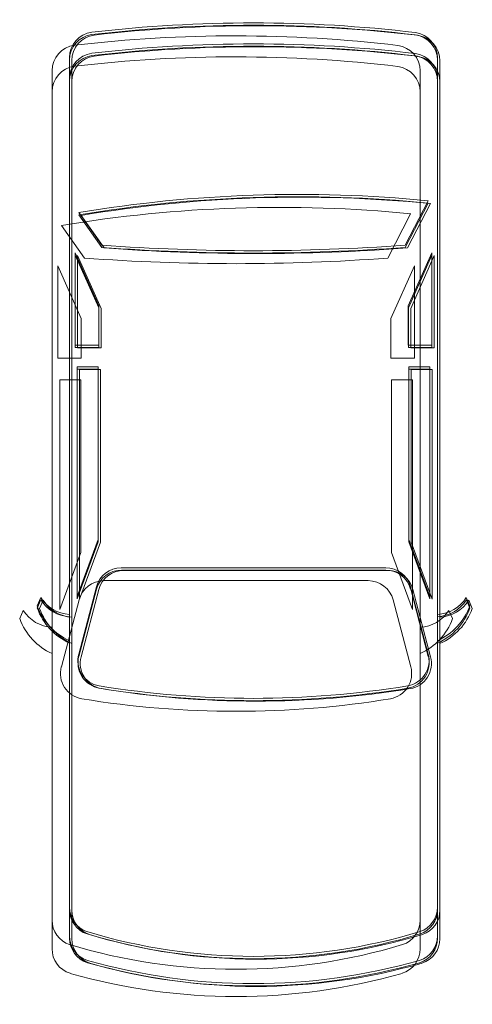
# Model space of a CAD drawing. Units: inches. Extents: x 79 to 8696167, y -3690578 to 147.
# Tile 10 of 10: x 8692662 to 8696167, y -3690578 to -3682952. Entities that reach past the tile are written whole.
import ezdxf

# ---------------------------------------------------------------- set-up
doc = ezdxf.new("R2010")
doc.units = ezdxf.units.IN
doc.header["$MEASUREMENT"] = 0
doc.layers.add('C-PKNG-VEHI', color=8, linetype='Continuous', lineweight=13)
doc.layers.add('PLUMBING FIXTURES', color=9, linetype='Continuous', lineweight=18)

# ---------------------------------------------------------------- blocks, each defined once
blk = doc.blocks.new('CAR')
at = {"layer": 'PLUMBING FIXTURES', "ltscale": 3}
for p, q in [((220804.47, -93720.06), (220804.47, -93547.3)), ((220876.86, -93720.06), (220876.86, -93547.35)), ((220870.5, -93584.17), (220875, -93575.44)), ((220810.83, -93584.17), (220806.31, -93577.76)), ((220810.23, -93596.08), (220805.58, -93585.68)), ((220805.58, -93585.68), (220805.58, -93603.85)), ((220871.11, -93596.08), (220875.75, -93585.68)), ((220875.75, -93585.68), (220875.75, -93603.85)), ((220810.23, -93603.85), (220810.23, -93596.08)), ((220871.11, -93603.85), (220871.11, -93596.08)), ((220805.58, -93603.85), (220810.23, -93603.85)), ((220875.75, -93603.85), (220871.11, -93603.85)), ((220805.99, -93608.09), (220810.13, -93608.09)), ((220805.99, -93653.29), (220805.99, -93608.09)), ((220810.13, -93608.09), (220810.13, -93642.08)), ((220875.35, -93608.09), (220871.21, -93608.09)), ((220871.21, -93608.09), (220871.21, -93642.08)), ((220875.35, -93653.29), (220875.35, -93608.09)), ((220810.13, -93642.08), (220805.99, -93653.29)), ((220871.21, -93642.08), (220875.35, -93653.29)), ((220814.66, -93647.63), (220866.67, -93647.63)), ((220806.3, -93664.61), (220809.78, -93651.39)), ((220875.03, -93664.61), (220871.56, -93651.39)), ((220798.82, -93653.49), (220798.11, -93655.1)), ((220882.52, -93653.49), (220883.22, -93655.1))]:
    blk.add_line(p, q, dxfattribs=at)
for centre, radius, start, end in [((220840.49, -93811.75), 271.3, 83.2311, 96.6925), ((220809.52, -93547.3), 5.05, 97.3566, 180), ((220871.81, -93547.35), 5.05, 360, 82.5593), ((220840.49, -93815.88), 271.3, 83.2311, 96.6925), ((220809.52, -93551.44), 5.05, 97.3566, 180), ((220871.81, -93551.49), 5.05, 360, 82.5593), ((220849.45, -93836.99), 262.8, 84.4202, 99.448), ((220840.67, -93184.08), 401.19, 265.7353, 274.2647), ((220814.66, -93652.68), 5.05, 90, 165.2564), ((220866.67, -93652.68), 5.05, 14.7436, 90), ((220809.44, -93651.03), 12.03, 199.7943, 245.6458), ((220804.88, -93649.65), 7.17, 212.3474, 266.7713), ((220876.46, -93649.65), 7.17, 273.2287, 327.6525), ((220871.9, -93651.03), 12.03, 294.3542, 340.2056), ((220811.18, -93665.89), 5.05, 165.2564, 260.0648), ((220870.15, -93665.89), 5.05, 279.9351, 14.7436), ((220840.67, -93484.81), 188.52, 260.7342, 279.2658), ((220809.52, -93714.44), 5.05, 180, 251.4636), ((220871.81, -93714.44), 5.05, 288.5363, 360), ((220809.52, -93720.06), 5.05, 180, 252.5507), ((220840.67, -93611.64), 112.45, 253.0675, 286.9325), ((220871.81, -93720.06), 5.05, 287.4493, 360), ((220840.67, -93610.47), 118.98, 254.0673, 285.9327)]:
    blk.add_arc(centre, radius, start, end, dxfattribs=at)

msp = doc.modelspace()

# ---------------------------------------------------------------- block references
at = {"layer": 'C-PKNG-VEHI', "xscale": 39.37007874015748, "yscale": 39.37007874015748, "zscale": 39.37007874015748}
for p in [(-42.305, -281.497), (-41.346, -299.491), (-23.357, -303.272), (-176.856, -381.833)]:
    msp.add_blockref('CAR', p, dxfattribs=at)

doc.saveas('drawing.dxf')
